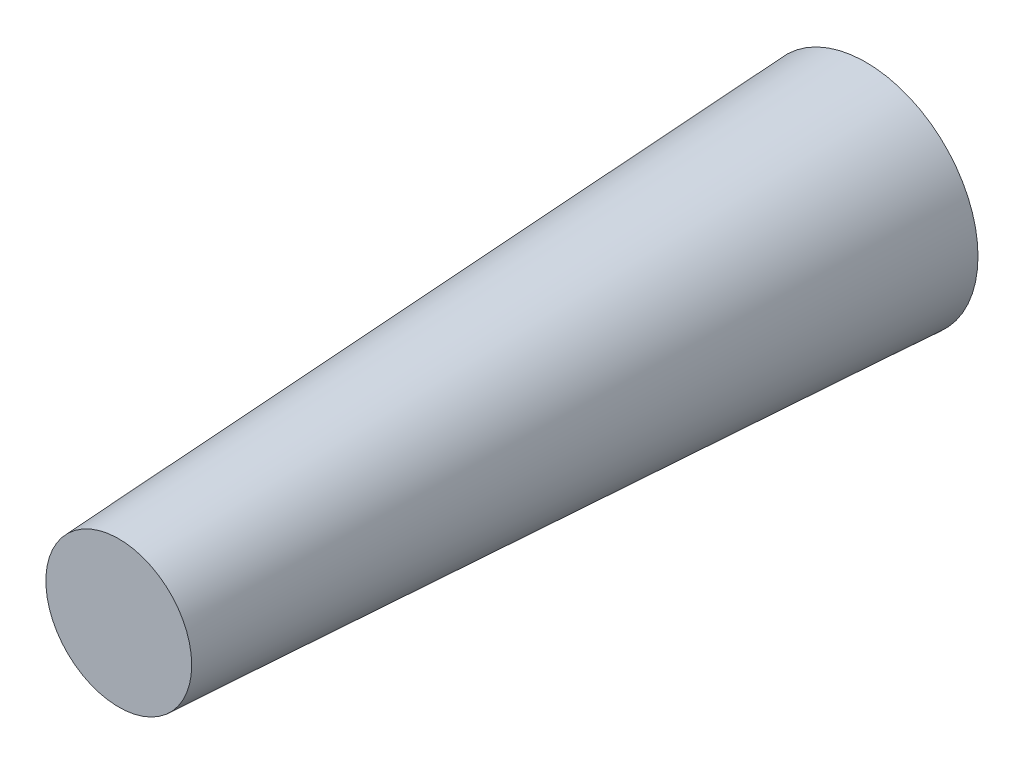
ISO-10303-21;
HEADER;
FILE_DESCRIPTION(('STEP AP214'),'2;1');
FILE_NAME('part.step','',(''),(''),'','','');
FILE_SCHEMA(('AUTOMOTIVE_DESIGN { 1 0 10303 214 1 1 1 1 }'));
ENDSEC;
DATA;
#1=APPLICATION_CONTEXT('core data for automotive mechanical design processes');
#2=APPLICATION_PROTOCOL_DEFINITION('international standard','automotive_design',2000,#1);
#3=PRODUCT_CONTEXT('',#1,'mechanical');
#4=PRODUCT('Part','Part','',(#3));
#5=PRODUCT_RELATED_PRODUCT_CATEGORY('part','',(#4));
#6=PRODUCT_DEFINITION_FORMATION('','',#4);
#7=PRODUCT_DEFINITION_CONTEXT('part definition',#1,'design');
#8=PRODUCT_DEFINITION('design','',#6,#7);
#9=PRODUCT_DEFINITION_SHAPE('','',#8);
#10=(LENGTH_UNIT() NAMED_UNIT(*) SI_UNIT(.MILLI.,.METRE.));
#11=(NAMED_UNIT(*) PLANE_ANGLE_UNIT() SI_UNIT($,.RADIAN.));
#12=(NAMED_UNIT(*) SI_UNIT($,.STERADIAN.) SOLID_ANGLE_UNIT());
#13=UNCERTAINTY_MEASURE_WITH_UNIT(LENGTH_MEASURE(1.E-05),#10,'distance_accuracy_value','');
#14=(GEOMETRIC_REPRESENTATION_CONTEXT(3) GLOBAL_UNCERTAINTY_ASSIGNED_CONTEXT((#13)) GLOBAL_UNIT_ASSIGNED_CONTEXT((#10,
#11,#12)) REPRESENTATION_CONTEXT('',''));
#15=CARTESIAN_POINT('',(0.,0.,0.));
#16=DIRECTION('',(0.,0.,1.));
#17=DIRECTION('',(1.,0.,0.));
#18=AXIS2_PLACEMENT_3D('',#15,#16,#17);
#19=CARTESIAN_POINT('',(0.,0.,0.));
#20=DIRECTION('',(0.,0.,-1.));
#21=DIRECTION('',(1.,0.,0.));
#22=AXIS2_PLACEMENT_3D('',#19,#20,#21);
#23=CONICAL_SURFACE('',#22,3.,0.05235987755983);
#24=CARTESIAN_POINT('',(0.,0.,20.));
#25=DIRECTION('',(0.,0.,1.));
#26=DIRECTION('',(1.,0.,0.));
#27=AXIS2_PLACEMENT_3D('',#24,#25,#26);
#28=CIRCLE('',#27,1.95184441433917);
#29=CARTESIAN_POINT('',(1.95184441433917,0.,20.));
#30=VERTEX_POINT('',#29);
#31=EDGE_CURVE('E10',#30,#30,#28,.T.);
#32=ORIENTED_EDGE('',*,*,#31,.F.);
#33=EDGE_LOOP('',(#32));
#34=FACE_BOUND('',#33,.T.);
#35=CARTESIAN_POINT('',(0.,0.,0.));
#36=DIRECTION('',(0.,0.,1.));
#37=DIRECTION('',(1.,0.,0.));
#38=AXIS2_PLACEMENT_3D('',#35,#36,#37);
#39=CIRCLE('',#38,3.);
#40=CARTESIAN_POINT('',(3.,0.,0.));
#41=VERTEX_POINT('',#40);
#42=EDGE_CURVE('E43',#41,#41,#39,.T.);
#43=ORIENTED_EDGE('',*,*,#42,.T.);
#44=EDGE_LOOP('',(#43));
#45=FACE_BOUND('',#44,.T.);
#46=ADVANCED_FACE('F40',(#34,#45),#23,.T.);
#47=CARTESIAN_POINT('',(0.,0.,20.));
#48=DIRECTION('',(0.,0.,1.));
#49=DIRECTION('',(1.,0.,0.));
#50=AXIS2_PLACEMENT_3D('',#47,#48,#49);
#51=PLANE('',#50);
#52=ORIENTED_EDGE('',*,*,#31,.T.);
#53=EDGE_LOOP('',(#52));
#54=FACE_BOUND('',#53,.T.);
#55=ADVANCED_FACE('F55',(#54),#51,.T.);
#56=CARTESIAN_POINT('',(0.,0.,0.));
#57=DIRECTION('',(0.,0.,1.));
#58=DIRECTION('',(1.,0.,0.));
#59=AXIS2_PLACEMENT_3D('',#56,#57,#58);
#60=PLANE('',#59);
#61=ORIENTED_EDGE('',*,*,#42,.F.);
#62=EDGE_LOOP('',(#61));
#63=FACE_BOUND('',#62,.T.);
#64=ADVANCED_FACE('F49',(#63),#60,.F.);
#65=CLOSED_SHELL('',(#46,#55,#64));
#66=MANIFOLD_SOLID_BREP('B2',#65);
#67=ADVANCED_BREP_SHAPE_REPRESENTATION('',(#18,#66),#14);
#68=SHAPE_DEFINITION_REPRESENTATION(#9,#67);
ENDSEC;
END-ISO-10303-21;
